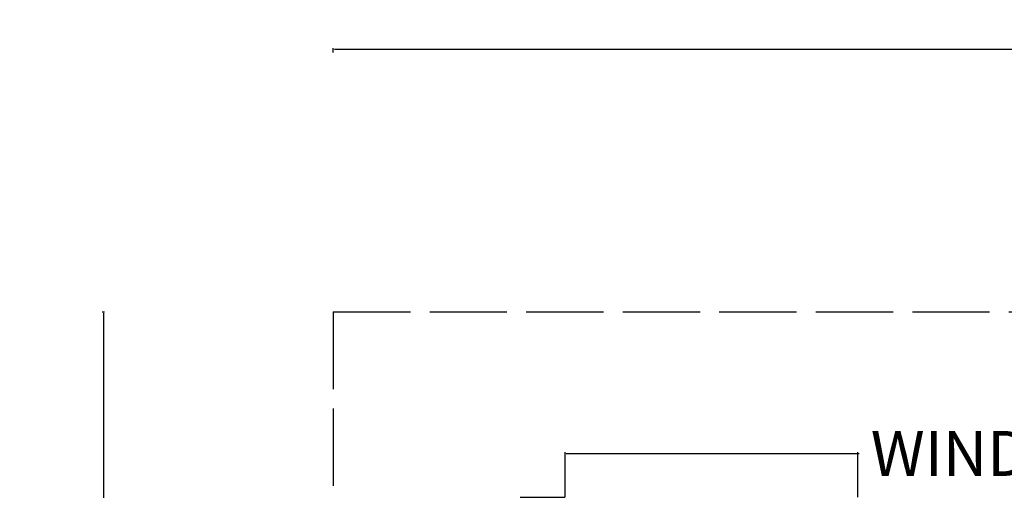
# Model space of a CAD drawing. Units: inches. Extents: x 1316 to 1777, y 813 to 1650.
# Tile 13 of 22: x 1316 to 1469, y 1576 to 1650. Entities that reach past the tile are written whole.
import ezdxf

# ---------------------------------------------------------------- set-up
doc = ezdxf.new("R2010")
doc.units = ezdxf.units.IN
doc.header["$MEASUREMENT"] = 0
doc.linetypes.add('ACAD_ISO02W100', pattern=[15, 12, -3])
doc.layers.add('A-ANNO-DIMS', color=2, linetype='Continuous', lineweight=18)
doc.layers.add('C-PROP', color=8, linetype='ACAD_ISO02W100', lineweight=25)
doc.styles.get("Standard").update_dxf_attribs({"font": 'arial.ttf'})
doc.dimstyles.get("Standard").update_dxf_attribs({"dimtxt": 7, "dimasz": 0.18, "dimexe": 0.18, "dimexo": 0.0625, "dimgap": 0.09, "dimtad": 0, "dimtih": 1, "dimtoh": 1, "dimzin": 0, "dimdsep": 46, "dimlunit": 3, "dimtxsty": 'Standard', "dimcen": 0.09, "dimadec": 0, "dimazin": 0, "dimtfac": 1, "dimtofl": 0, "dimtmove": 0, "dimatfit": 3, "dimfxl": 1, "dimtolj": 1, "dimtzin": 0, "dimarcsym": 0})

# ---------------------------------------------------------------- blocks, each defined once
blk = doc.blocks.new('*D22')
at = {"layer": 'A-ANNO-DIMS', "color": 0, "lineweight": -2, "transparency": 16777216}
for p, q in [((1364.4, 1644.46), (1364.4, 1645.13)), ((1364.58, 1644.95), (1532.29, 1644.95)), ((1724.22, 1644.95), (1556.51, 1644.95)), ((1724.4, 1644.46), (1724.4, 1645.13))]:
    blk.add_line(p, q, dxfattribs=at)
at = {"layer": 'A-ANNO-DIMS', "color": 0, "transparency": 16777216}
for points in [[(1364.58, 1644.98), (1364.58, 1644.92), (1364.4, 1644.95)], [(1724.22, 1644.98), (1724.22, 1644.92), (1724.4, 1644.95)]]:
    blk.add_solid(points, dxfattribs=at)
at = {"layer": 'Defpoints', "color": 0, "transparency": 16777216}
for p in [(1724.4, 1644.95), (1364.4, 1644.4), (1724.4, 1644.4)]:
    blk.add_point(p, dxfattribs=at)
at = {"layer": 'A-ANNO-DIMS', "color": 0, "transparency": 16777216, "insert": (1544.4, 1644.95), "char_height": 7, "attachment_point": 5}
blk.add_mtext('\\A1;30\'-0"', dxfattribs=at)
blk = doc.blocks.new('*D23')
at = {"layer": 'A-ANNO-DIMS', "color": 0, "lineweight": -2, "transparency": 16777216}
for p, q in [((1328.47, 1604.17), (1328.87, 1604.17)), ((1328.69, 1603.99), (1328.69, 1282.59)), ((1328.69, 953.87), (1328.69, 1275.27)), ((1328.47, 953.69), (1328.87, 953.69))]:
    blk.add_line(p, q, dxfattribs=at)
at = {"layer": 'A-ANNO-DIMS', "color": 0, "transparency": 16777216}
for points in [[(1328.66, 1603.99), (1328.72, 1603.99), (1328.69, 1604.17)], [(1328.66, 953.87), (1328.72, 953.87), (1328.69, 953.69)]]:
    blk.add_solid(points, dxfattribs=at)
at = {"layer": 'Defpoints', "color": 0, "transparency": 16777216}
for p in [(1328.4, 1604.17), (1328.4, 953.69), (1328.69, 953.69)]:
    blk.add_point(p, dxfattribs=at)
at = {"layer": 'A-ANNO-DIMS', "color": 0, "transparency": 16777216, "insert": (1328.69, 1278.93), "char_height": 7, "width": 24.3281, "attachment_point": 5}
blk.add_mtext('\\A1;47\'-0"', dxfattribs=at)
blk = doc.blocks.new('*D34')
at = {"layer": 'A-ANNO-DIMS', "color": 0, "lineweight": -2, "transparency": 16777216}
for p, q in [((1400.44, 1575.43), (1400.44, 1582.38)), ((1400.62, 1582.2), (1445.77, 1582.2)), ((1445.95, 1575.43), (1445.95, 1582.38)), ((1445.95, 1582.2), (1446.13, 1582.2))]:
    blk.add_line(p, q, dxfattribs=at)
at = {"layer": 'A-ANNO-DIMS', "color": 0, "transparency": 16777216}
for points in [[(1400.62, 1582.23), (1400.62, 1582.17), (1400.44, 1582.2)], [(1445.77, 1582.23), (1445.77, 1582.17), (1445.95, 1582.2)]]:
    blk.add_solid(points, dxfattribs=at)
at = {"layer": 'Defpoints', "color": 0, "transparency": 16777216}
for p in [(1445.95, 1582.2), (1400.44, 1575.37), (1445.95, 1575.37)]:
    blk.add_point(p, dxfattribs=at)
at = {"layer": 'A-ANNO-DIMS', "color": 0, "transparency": 16777216, "insert": (1498.67, 1582.2), "char_height": 7, "attachment_point": 5}
blk.add_mtext('\\A1;WINDOW 3\'-9 1/2" TYP.', dxfattribs=at)
blk = doc.blocks.new('*D35')
at = {"layer": 'A-ANNO-DIMS', "color": 0, "lineweight": -2, "transparency": 16777216}
for p, q in [((1400.38, 1575.37), (1393.44, 1575.37)), ((1393.62, 1575.19), (1393.62, 1574.53)), ((1393.62, 1566.55), (1393.62, 1567.21)), ((1400.38, 1566.37), (1393.44, 1566.37))]:
    blk.add_line(p, q, dxfattribs=at)
at = {"layer": 'A-ANNO-DIMS', "color": 0, "transparency": 16777216}
for points in [[(1393.59, 1575.19), (1393.65, 1575.19), (1393.62, 1575.37)], [(1393.59, 1566.55), (1393.65, 1566.55), (1393.62, 1566.37)]]:
    blk.add_solid(points, dxfattribs=at)
at = {"layer": 'Defpoints', "color": 0, "transparency": 16777216}
for p in [(1393.62, 1575.37), (1400.44, 1575.37), (1400.44, 1566.37)]:
    blk.add_point(p, dxfattribs=at)
at = {"layer": 'A-ANNO-DIMS', "color": 0, "transparency": 16777216, "insert": (1393.62, 1570.87), "char_height": 7, "attachment_point": 5}
blk.add_mtext('\\A1;0\'-9" TYP.', dxfattribs=at)

msp = doc.modelspace()

# ---------------------------------------------------------------- linework, layer by layer
at = {"layer": 'C-PROP'}
for q in [(1724.399, 1604.173), (1364.399, 953.689)]:
    msp.add_line((1364.399, 1604.173), q, dxfattribs=at)

# ---------------------------------------------------------------- dimensions: what is measured, and where the dimension line sits
at = {"layer": 'A-ANNO-DIMS'}
for base, p1, p2, text, override, picture, middle in [((1724.399, 1644.949), (1364.399, 1644.396), (1724.399, 1644.396), '30\'-0"', {"dimclrd": 0, "dimclre": 0, "dimclrt": 0}, '*D22', (1544.399, 1644.949)), ((1445.955, 1582.196), (1400.445, 1575.369), (1445.955, 1575.369), 'WINDOW <> TYP.', {"dimdec": 1, "dimlfac": 1, "dimrnd": 0, "dimzin": 1, "dimdsep": 46, "dimlunit": 4, "dimfrac": 2}, '*D34', (1498.67, 1582.196))]:
    dim = msp.add_linear_dim(base=base, p1=p1, p2=p2, text=text, dimstyle='Standard', override=override, dxfattribs=at)
    dim.commit()
    dim.dimension.update_dxf_attribs({"geometry": picture, "text_midpoint": middle})
for base, p1, p2, text, override, picture, middle in [((1328.686, 953.689), (1328.404, 1604.173), (1328.404, 953.689), '47\'-0"', {"dimclrd": 0, "dimclre": 0, "dimclrt": 0}, '*D23', (1328.686, 1278.931)), ((1393.618, 1575.369), (1400.445, 1566.369), (1400.445, 1575.369), '<> TYP.', {"dimdec": 1, "dimlfac": 1, "dimrnd": 0, "dimzin": 1, "dimdsep": 46, "dimlunit": 4, "dimfrac": 2}, '*D35', (1393.618, 1570.869))]:
    dim = msp.add_linear_dim(base=base, p1=p1, p2=p2, angle=90, text=text, dimstyle='Standard', override=override, dxfattribs=at)
    dim.commit()
    dim.dimension.update_dxf_attribs({"geometry": picture, "text_midpoint": middle})

doc.saveas('drawing.dxf')
